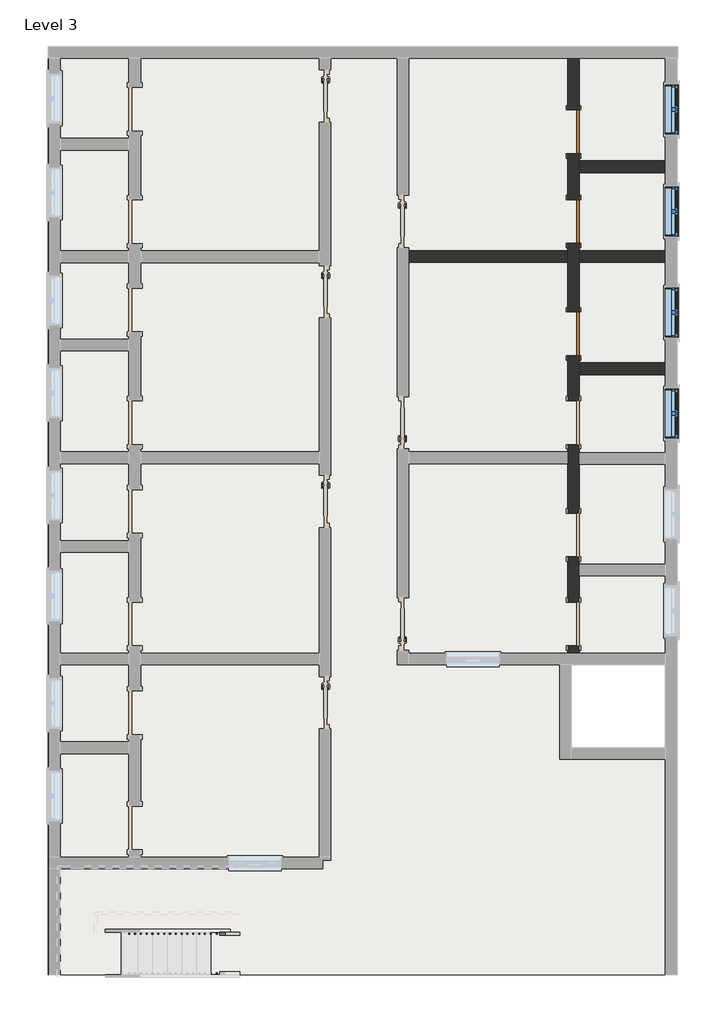
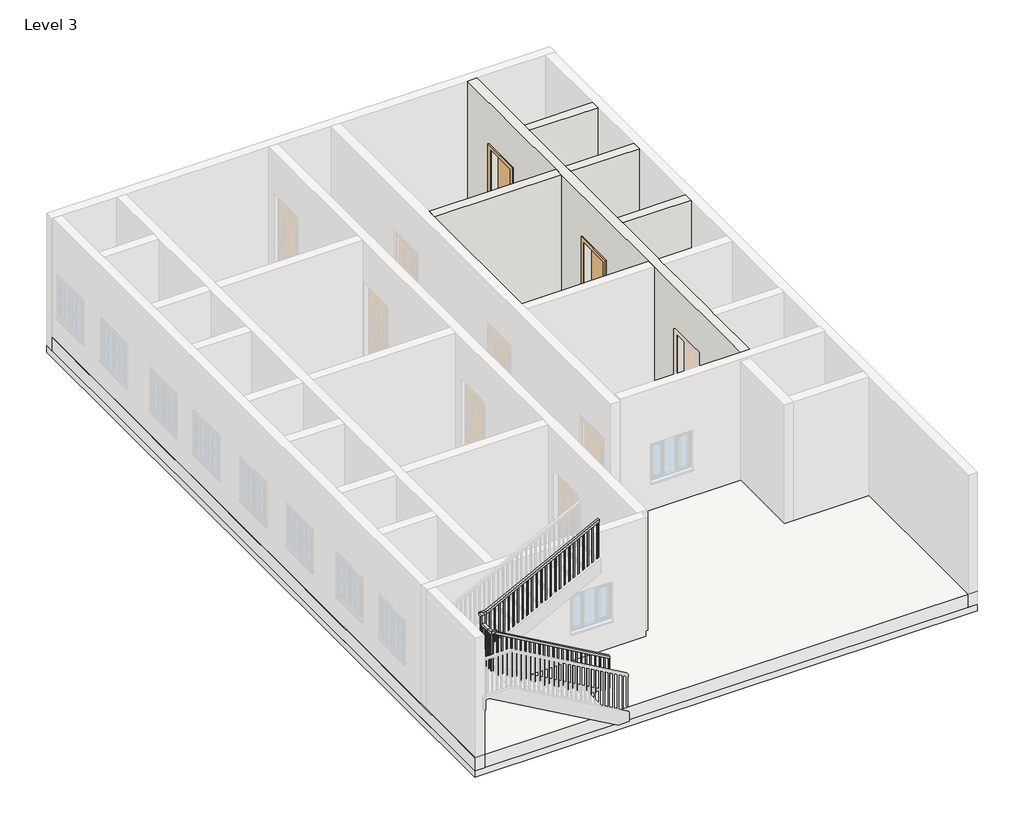
# One storey, part 2 of 4: 5 walls, 4 windows, 3 doors, 1 railing, 1 roof, 1 slab.
"""IFC4 building model written with IfcOpenShell, lengths in millimetres."""

from ifc_helpers import new_model, si_unit, frame, origin, place, context, project, spatial, polyline, outline, extrude, faceted_brep, transform, mapped, element, save
from components import door_53b1b562, window_c29befe5

model = new_model("IFC4")

# Units and contexts
model_context = context("Model", 3, world=origin())
ifc_project = project(units=[si_unit("LENGTHUNIT", "METRE", prefix="MILLI")], contexts=[model_context])

# Site, building, storey
site = spatial("IfcSite", under=ifc_project)
building = spatial("IfcBuilding", under=site)
storey = spatial("IfcBuildingStorey", under=building, Name="Level 3", Elevation=6096.0)

# Doors
placement = place(None, origin())
door_shape = door_53b1b562(model_context)
element("IfcDoor", 1, ObjectType="Single-Flush : 30\" x 80\"", at=placement, inside=storey, context=model_context, shape_type="MappedRepresentation", body=[
    mapped(door_shape, transform((2695.5891134, 6512.9399728, 6096.0), x_axis=(0.0, 1.0, 0.0), y_axis=(-1.0, 0.0, 0.0), z_axis=(0.0, 0.0, 1.0))),
])
element("IfcDoor", 2, ObjectType="Single-Flush : 30\" x 80\"", at=placement, inside=storey, context=model_context, shape_type="MappedRepresentation", body=[
    mapped(door_shape, transform((2695.5891134, 4950.8399728, 6096.0), x_axis=(0.0, 1.0, 0.0), y_axis=(-1.0, 0.0, 0.0), z_axis=(0.0, 0.0, 1.0))),
])
element("IfcDoor", 3, ObjectType="Single-Flush : 30\" x 80\"", at=placement, inside=storey, context=model_context, shape_type="MappedRepresentation", body=[
    mapped(door_shape, transform((2695.5891134, 2995.0399728, 6096.0), x_axis=(0.0, 1.0, 0.0), y_axis=(-1.0, 0.0, 0.0), z_axis=(0.0, 0.0, 1.0))),
])

# Railing
element("IfcRailing", 4, ObjectType="Handrail - Rectangular", at=placement, inside=storey, context=model_context, shape_type="SolidModel", body=[
    faceted_brep([(-3117.2664982, -7482.4600272, 7155.5428571), (-3117.2664982, -7482.4600272, 7097.0339009), (-3117.2664982, -7431.6600272, 7097.0339009), (-3117.2664982, -7431.6600272, 7155.5428571), (-5581.0664982, -7482.4600272, 8563.4285714), (-5631.8664982, -7482.4600272, 8533.9481866), (-5631.8664982, -7431.6600272, 8533.9481866), (-5581.0664982, -7431.6600272, 8563.4285714), (-5581.0664982, -7482.4600272, 8606.9714286), (-5631.8664982, -7482.4600272, 8556.1714286), (-5631.8664982, -7431.6600272, 8556.1714286), (-5581.0664982, -7431.6600272, 8606.9714286), (-5708.0664982, -7482.4600272, 8606.9714286), (-5708.0664982, -7482.4600272, 8556.1714286), (-5657.2664982, -7431.6600272, 8556.1714286), (-5657.2664982, -7431.6600272, 8606.9714286), (-5708.0664982, -7355.4600272, 8606.9714286), (-5708.0664982, -7355.4600272, 8556.1714286), (-5657.2664982, -7355.4600272, 8556.1714286), (-5657.2664982, -7355.4600272, 8606.9714286), (-5708.0664982, -7152.2600272, 8606.9714286), (-5708.0664982, -7101.4600272, 8556.1714286), (-5657.2664982, -7101.4600272, 8556.1714286), (-5657.2664982, -7152.2600272, 8606.9714286), (-5708.0664982, -7152.2600272, 8791.3028571), (-5708.0664982, -7101.4600272, 8740.5028571), (-5657.2664982, -7101.4600272, 8740.5028571), (-5657.2664982, -7152.2600272, 8791.3028571), (-5708.0664982, -7025.2600272, 8791.3028571), (-5708.0664982, -7025.2600272, 8740.5028571), (-5657.2664982, -7076.0600272, 8740.5028571), (-5657.2664982, -7076.0600272, 8791.3028571), (-5581.0664982, -7025.2600272, 8791.3028571), (-5568.769124, -7025.2600272, 8740.5028571), (-5568.769124, -7076.0600272, 8740.5028571), (-5581.0664982, -7076.0600272, 8791.3028571), (-3117.2664982, -7025.2600272, 10058.4), (-3117.2664982, -7076.0600272, 10058.4), (-3117.2664982, -7076.0600272, 10001.2756361), (-3117.2664982, -7025.2600272, 10001.2756361)], [[[0, 1, 2, 3]], [[1, 0, 4, 5]], [[2, 1, 5, 6]], [[3, 2, 6, 7]], [[0, 3, 7, 4]], [[5, 4, 8, 9]], [[6, 5, 9, 10]], [[7, 6, 10, 11]], [[4, 7, 11, 8]], [[9, 8, 12, 13]], [[10, 9, 13, 14]], [[11, 10, 14, 15]], [[8, 11, 15, 12]], [[13, 12, 16, 17]], [[14, 13, 17, 18]], [[15, 14, 18, 19]], [[12, 15, 19, 16]], [[17, 16, 20, 21]], [[18, 17, 21, 22]], [[19, 18, 22, 23]], [[16, 19, 23, 20]], [[21, 20, 24, 25]], [[22, 21, 25, 26]], [[23, 22, 26, 27]], [[20, 23, 27, 24]], [[25, 24, 28, 29]], [[26, 25, 29, 30]], [[27, 26, 30, 31]], [[24, 27, 31, 28]], [[29, 28, 32, 33]], [[30, 29, 33, 34]], [[31, 30, 34, 35]], [[28, 31, 35, 32]], [[36, 37, 38, 39]], [[33, 32, 36, 39]], [[34, 33, 39, 38]], [[35, 34, 38, 37]], [[32, 35, 37, 36]]]),
    extrude(outline(polyline([(9993.1113504, -3133.1414982), (9983.3142076, -3152.1914982), (8998.8571429, -3152.1914982), (8998.8571429, -3133.1414982), (9993.1113504, -3133.1414982)])), frame((0.0, -7060.1850272, 0.0), z_axis=(0.0, 1.0, 0.0), x_axis=(0.0, 0.0, 1.0)), (0.0, 0.0, 1.0), 19.05),
    extrude(outline(polyline([(9940.8599218, -3234.7414982), (9931.062779, -3253.7914982), (8998.8571429, -3253.7914982), (8998.8571429, -3234.7414982), (9940.8599218, -3234.7414982)])), frame((0.0, -7060.1850272, 0.0), z_axis=(0.0, 1.0, 0.0), x_axis=(0.0, 0.0, 1.0)), (0.0, 0.0, 1.0), 19.05),
    extrude(outline(polyline([(9888.6084933, -3336.3414982), (9878.8113504, -3355.3914982), (8998.8571429, -3355.3914982), (8998.8571429, -3336.3414982), (9888.6084933, -3336.3414982)])), frame((0.0, -7060.1850272, 0.0), z_axis=(0.0, 1.0, 0.0), x_axis=(0.0, 0.0, 1.0)), (0.0, 0.0, 1.0), 19.05),
    extrude(outline(polyline([(9836.3570647, -3437.9414982), (9826.5599218, -3456.9914982), (8853.7142857, -3456.9914982), (8853.7142857, -3437.9414982), (9836.3570647, -3437.9414982)])), frame((0.0, -7060.1850272, 0.0), z_axis=(0.0, 1.0, 0.0), x_axis=(0.0, 0.0, 1.0)), (0.0, 0.0, 1.0), 19.05),
    extrude(outline(polyline([(9784.1056361, -3539.5414982), (9774.3084933, -3558.5914982), (8853.7142857, -3558.5914982), (8853.7142857, -3539.5414982), (9784.1056361, -3539.5414982)])), frame((0.0, -7060.1850272, 0.0), z_axis=(0.0, 1.0, 0.0), x_axis=(0.0, 0.0, 1.0)), (0.0, 0.0, 1.0), 19.05),
    extrude(outline(polyline([(9731.8542076, -3641.1414982), (9722.0570647, -3660.1914982), (8708.5714286, -3660.1914982), (8708.5714286, -3641.1414982), (9731.8542076, -3641.1414982)])), frame((0.0, -7060.1850272, 0.0), z_axis=(0.0, 1.0, 0.0), x_axis=(0.0, 0.0, 1.0)), (0.0, 0.0, 1.0), 19.05),
    extrude(outline(polyline([(9679.602779, -3742.7414982), (9669.8056361, -3761.7914982), (8708.5714286, -3761.7914982), (8708.5714286, -3742.7414982), (9679.602779, -3742.7414982)])), frame((0.0, -7060.1850272, 0.0), z_axis=(0.0, 1.0, 0.0), x_axis=(0.0, 0.0, 1.0)), (0.0, 0.0, 1.0), 19.05),
    extrude(outline(polyline([(9627.3513504, -3844.3414982), (9617.5542076, -3863.3914982), (8708.5714286, -3863.3914982), (8708.5714286, -3844.3414982), (9627.3513504, -3844.3414982)])), frame((0.0, -7060.1850272, 0.0), z_axis=(0.0, 1.0, 0.0), x_axis=(0.0, 0.0, 1.0)), (0.0, 0.0, 1.0), 19.05),
    extrude(outline(polyline([(9575.0999218, -3945.9414982), (9565.302779, -3964.9914982), (8708.5714286, -3964.9914982), (8708.5714286, -3945.9414982), (9575.0999218, -3945.9414982)])), frame((0.0, -7060.1850272, 0.0), z_axis=(0.0, 1.0, 0.0), x_axis=(0.0, 0.0, 1.0)), (0.0, 0.0, 1.0), 19.05),
    extrude(outline(polyline([(9522.8484933, -4047.5414982), (9513.0513504, -4066.5914982), (8708.5714286, -4066.5914982), (8708.5714286, -4047.5414982), (9522.8484933, -4047.5414982)])), frame((0.0, -7060.1850272, 0.0), z_axis=(0.0, 1.0, 0.0), x_axis=(0.0, 0.0, 1.0)), (0.0, 0.0, 1.0), 19.05),
    extrude(outline(polyline([(9470.5970647, -4149.1414982), (9460.7999218, -4168.1914982), (8563.4285714, -4168.1914982), (8563.4285714, -4149.1414982), (9470.5970647, -4149.1414982)])), frame((0.0, -7060.1850272, 0.0), z_axis=(0.0, 1.0, 0.0), x_axis=(0.0, 0.0, 1.0)), (0.0, 0.0, 1.0), 19.05),
    extrude(outline(polyline([(9418.3456361, -4250.7414982), (9408.5484933, -4269.7914982), (8563.4285714, -4269.7914982), (8563.4285714, -4250.7414982), (9418.3456361, -4250.7414982)])), frame((0.0, -7060.1850272, 0.0), z_axis=(0.0, 1.0, 0.0), x_axis=(0.0, 0.0, 1.0)), (0.0, 0.0, 1.0), 19.05),
    extrude(outline(polyline([(9366.0942076, -4352.3414982), (9356.2970647, -4371.3914982), (8563.4285714, -4371.3914982), (8563.4285714, -4352.3414982), (9366.0942076, -4352.3414982)])), frame((0.0, -7060.1850272, 0.0), z_axis=(0.0, 1.0, 0.0), x_axis=(0.0, 0.0, 1.0)), (0.0, 0.0, 1.0), 19.05),
    extrude(outline(polyline([(9313.842779, -4453.9414982), (9304.0456361, -4472.9914982), (8418.2857143, -4472.9914982), (8418.2857143, -4453.9414982), (9313.842779, -4453.9414982)])), frame((0.0, -7060.1850272, 0.0), z_axis=(0.0, 1.0, 0.0), x_axis=(0.0, 0.0, 1.0)), (0.0, 0.0, 1.0), 19.05),
    extrude(outline(polyline([(9261.5913504, -4555.5414982), (9251.7942076, -4574.5914982), (8418.2857143, -4574.5914982), (8418.2857143, -4555.5414982), (9261.5913504, -4555.5414982)])), frame((0.0, -7060.1850272, 0.0), z_axis=(0.0, 1.0, 0.0), x_axis=(0.0, 0.0, 1.0)), (0.0, 0.0, 1.0), 19.05),
    extrude(outline(polyline([(9209.3399218, -4657.1414982), (9199.542779, -4676.1914982), (8273.1428571, -4676.1914982), (8273.1428571, -4657.1414982), (9209.3399218, -4657.1414982)])), frame((0.0, -7060.1850272, 0.0), z_axis=(0.0, 1.0, 0.0), x_axis=(0.0, 0.0, 1.0)), (0.0, 0.0, 1.0), 19.05),
    extrude(outline(polyline([(9157.0884933, -4758.7414982), (9147.2913504, -4777.7914982), (8273.1428571, -4777.7914982), (8273.1428571, -4758.7414982), (9157.0884933, -4758.7414982)])), frame((0.0, -7060.1850272, 0.0), z_axis=(0.0, 1.0, 0.0), x_axis=(0.0, 0.0, 1.0)), (0.0, 0.0, 1.0), 19.05),
    extrude(outline(polyline([(9104.8370647, -4860.3414982), (9095.0399218, -4879.3914982), (8273.1428571, -4879.3914982), (8273.1428571, -4860.3414982), (9104.8370647, -4860.3414982)])), frame((0.0, -7060.1850272, 0.0), z_axis=(0.0, 1.0, 0.0), x_axis=(0.0, 0.0, 1.0)), (0.0, 0.0, 1.0), 19.05),
    extrude(outline(polyline([(9052.5856361, -4961.9414982), (9042.7884933, -4980.9914982), (8128.0, -4980.9914982), (8128.0, -4961.9414982), (9052.5856361, -4961.9414982)])), frame((0.0, -7060.1850272, 0.0), z_axis=(0.0, 1.0, 0.0), x_axis=(0.0, 0.0, 1.0)), (0.0, 0.0, 1.0), 19.05),
    extrude(outline(polyline([(9000.3342076, -5063.5414982), (8990.5370647, -5082.5914982), (8128.0, -5082.5914982), (8128.0, -5063.5414982), (9000.3342076, -5063.5414982)])), frame((0.0, -7060.1850272, 0.0), z_axis=(0.0, 1.0, 0.0), x_axis=(0.0, 0.0, 1.0)), (0.0, 0.0, 1.0), 19.05),
    extrude(outline(polyline([(8948.082779, -5165.1414982), (8938.2856361, -5184.1914982), (7982.8571429, -5184.1914982), (7982.8571429, -5165.1414982), (8948.082779, -5165.1414982)])), frame((0.0, -7060.1850272, 0.0), z_axis=(0.0, 1.0, 0.0), x_axis=(0.0, 0.0, 1.0)), (0.0, 0.0, 1.0), 19.05),
    extrude(outline(polyline([(8895.8313504, -5266.7414982), (8886.0342076, -5285.7914982), (7982.8571429, -5285.7914982), (7982.8571429, -5266.7414982), (8895.8313504, -5266.7414982)])), frame((0.0, -7060.1850272, 0.0), z_axis=(0.0, 1.0, 0.0), x_axis=(0.0, 0.0, 1.0)), (0.0, 0.0, 1.0), 19.05),
    extrude(outline(polyline([(8843.5799218, -5368.3414982), (8833.782779, -5387.3914982), (7982.8571429, -5387.3914982), (7982.8571429, -5368.3414982), (8843.5799218, -5368.3414982)])), frame((0.0, -7060.1850272, 0.0), z_axis=(0.0, 1.0, 0.0), x_axis=(0.0, 0.0, 1.0)), (0.0, 0.0, 1.0), 19.05),
    extrude(outline(polyline([(8791.3284933, -5469.9414982), (8781.5313504, -5488.9914982), (7837.7142857, -5488.9914982), (7837.7142857, -5469.9414982), (8791.3284933, -5469.9414982)])), frame((0.0, -7060.1850272, 0.0), z_axis=(0.0, 1.0, 0.0), x_axis=(0.0, 0.0, 1.0)), (0.0, 0.0, 1.0), 19.05),
    extrude(outline(polyline([(8739.0770647, -5571.5414982), (8729.2799218, -5590.5914982), (7837.7142857, -5590.5914982), (7837.7142857, -5571.5414982), (8739.0770647, -5571.5414982)])), frame((0.0, -7060.1850272, 0.0), z_axis=(0.0, 1.0, 0.0), x_axis=(0.0, 0.0, 1.0)), (0.0, 0.0, 1.0), 19.05),
    extrude(outline(polyline([(-5673.1414982, -7161.7850272), (-5692.1914982, -7161.7850272), (-5692.1914982, -7142.7350272), (-5673.1414982, -7142.7350272), (-5673.1414982, -7161.7850272)])), frame((0.0, 0.0, 7692.5714286), z_axis=(0.0, 0.0, 1.0), x_axis=(1.0, 0.0, 0.0)), (0.0, 0.0, 1.0), 863.6),
    extrude(outline(polyline([(-5673.1414982, -7263.3850272), (-5692.1914982, -7263.3850272), (-5692.1914982, -7244.3350272), (-5673.1414982, -7244.3350272), (-5673.1414982, -7263.3850272)])), frame((0.0, 0.0, 7692.5714286), z_axis=(0.0, 0.0, 1.0), x_axis=(1.0, 0.0, 0.0)), (0.0, 0.0, 1.0), 863.6),
    extrude(outline(polyline([(-5673.1414982, -7364.9850272), (-5692.1914982, -7364.9850272), (-5692.1914982, -7345.9350272), (-5673.1414982, -7345.9350272), (-5673.1414982, -7364.9850272)])), frame((0.0, 0.0, 7692.5714286), z_axis=(0.0, 0.0, 1.0), x_axis=(1.0, 0.0, 0.0)), (0.0, 0.0, 1.0), 863.6),
    extrude(outline(polyline([(-5647.7414982, -7447.5350272), (-5647.7414982, -7466.5850272), (-5666.7914982, -7466.5850272), (-5666.7914982, -7447.5350272), (-5647.7414982, -7447.5350272)])), frame((0.0, 0.0, 7692.5714286), z_axis=(0.0, 0.0, 1.0), x_axis=(1.0, 0.0, 0.0)), (0.0, 0.0, 1.0), 863.6),
    extrude(outline(polyline([(8484.9624723, -5546.1414982), (8495.8481866, -5565.1914982), (7547.4285714, -5565.1914982), (7547.4285714, -5546.1414982), (8484.9624723, -5546.1414982)])), frame((0.0, -7466.5850272, 0.0), z_axis=(0.0, 1.0, 0.0), x_axis=(0.0, 0.0, 1.0)), (0.0, 0.0, 1.0), 19.05),
    extrude(outline(polyline([(8426.9053295, -5444.5414982), (8437.7910438, -5463.5914982), (7547.4285714, -5463.5914982), (7547.4285714, -5444.5414982), (8426.9053295, -5444.5414982)])), frame((0.0, -7466.5850272, 0.0), z_axis=(0.0, 1.0, 0.0), x_axis=(0.0, 0.0, 1.0)), (0.0, 0.0, 1.0), 19.05),
    extrude(outline(polyline([(8368.8481866, -5342.9414982), (8379.7339009, -5361.9914982), (7402.2857143, -5361.9914982), (7402.2857143, -5342.9414982), (8368.8481866, -5342.9414982)])), frame((0.0, -7466.5850272, 0.0), z_axis=(0.0, 1.0, 0.0), x_axis=(0.0, 0.0, 1.0)), (0.0, 0.0, 1.0), 19.05),
    extrude(outline(polyline([(8310.7910438, -5241.3414982), (8321.6767581, -5260.3914982), (7402.2857143, -5260.3914982), (7402.2857143, -5241.3414982), (8310.7910438, -5241.3414982)])), frame((0.0, -7466.5850272, 0.0), z_axis=(0.0, 1.0, 0.0), x_axis=(0.0, 0.0, 1.0)), (0.0, 0.0, 1.0), 19.05),
    extrude(outline(polyline([(8252.7339009, -5139.7414982), (8263.6196152, -5158.7914982), (7402.2857143, -5158.7914982), (7402.2857143, -5139.7414982), (8252.7339009, -5139.7414982)])), frame((0.0, -7466.5850272, 0.0), z_axis=(0.0, 1.0, 0.0), x_axis=(0.0, 0.0, 1.0)), (0.0, 0.0, 1.0), 19.05),
    extrude(outline(polyline([(8194.6767581, -5038.1414982), (8205.5624723, -5057.1914982), (7257.1428571, -5057.1914982), (7257.1428571, -5038.1414982), (8194.6767581, -5038.1414982)])), frame((0.0, -7466.5850272, 0.0), z_axis=(0.0, 1.0, 0.0), x_axis=(0.0, 0.0, 1.0)), (0.0, 0.0, 1.0), 19.05),
    extrude(outline(polyline([(8136.6196152, -4936.5414982), (8147.5053295, -4955.5914982), (7257.1428571, -4955.5914982), (7257.1428571, -4936.5414982), (8136.6196152, -4936.5414982)])), frame((0.0, -7466.5850272, 0.0), z_axis=(0.0, 1.0, 0.0), x_axis=(0.0, 0.0, 1.0)), (0.0, 0.0, 1.0), 19.05),
    extrude(outline(polyline([(8078.5624723, -4834.9414982), (8089.4481866, -4853.9914982), (7112.0, -4853.9914982), (7112.0, -4834.9414982), (8078.5624723, -4834.9414982)])), frame((0.0, -7466.5850272, 0.0), z_axis=(0.0, 1.0, 0.0), x_axis=(0.0, 0.0, 1.0)), (0.0, 0.0, 1.0), 19.05),
    extrude(outline(polyline([(8020.5053295, -4733.3414982), (8031.3910438, -4752.3914982), (7112.0, -4752.3914982), (7112.0, -4733.3414982), (8020.5053295, -4733.3414982)])), frame((0.0, -7466.5850272, 0.0), z_axis=(0.0, 1.0, 0.0), x_axis=(0.0, 0.0, 1.0)), (0.0, 0.0, 1.0), 19.05),
    extrude(outline(polyline([(7962.4481866, -4631.7414982), (7973.3339009, -4650.7914982), (7112.0, -4650.7914982), (7112.0, -4631.7414982), (7962.4481866, -4631.7414982)])), frame((0.0, -7466.5850272, 0.0), z_axis=(0.0, 1.0, 0.0), x_axis=(0.0, 0.0, 1.0)), (0.0, 0.0, 1.0), 19.05),
    extrude(outline(polyline([(7904.3910438, -4530.1414982), (7915.2767581, -4549.1914982), (6966.8571429, -4549.1914982), (6966.8571429, -4530.1414982), (7904.3910438, -4530.1414982)])), frame((0.0, -7466.5850272, 0.0), z_axis=(0.0, 1.0, 0.0), x_axis=(0.0, 0.0, 1.0)), (0.0, 0.0, 1.0), 19.05),
    extrude(outline(polyline([(7846.3339009, -4428.5414982), (7857.2196152, -4447.5914982), (6966.8571429, -4447.5914982), (6966.8571429, -4428.5414982), (7846.3339009, -4428.5414982)])), frame((0.0, -7466.5850272, 0.0), z_axis=(0.0, 1.0, 0.0), x_axis=(0.0, 0.0, 1.0)), (0.0, 0.0, 1.0), 19.05),
    extrude(outline(polyline([(7788.2767581, -4326.9414982), (7799.1624723, -4345.9914982), (6821.7142857, -4345.9914982), (6821.7142857, -4326.9414982), (7788.2767581, -4326.9414982)])), frame((0.0, -7466.5850272, 0.0), z_axis=(0.0, 1.0, 0.0), x_axis=(0.0, 0.0, 1.0)), (0.0, 0.0, 1.0), 19.05),
    extrude(outline(polyline([(7730.2196152, -4225.3414982), (7741.1053295, -4244.3914982), (6821.7142857, -4244.3914982), (6821.7142857, -4225.3414982), (7730.2196152, -4225.3414982)])), frame((0.0, -7466.5850272, 0.0), z_axis=(0.0, 1.0, 0.0), x_axis=(0.0, 0.0, 1.0)), (0.0, 0.0, 1.0), 19.05),
    extrude(outline(polyline([(7672.1624723, -4123.7414982), (7683.0481866, -4142.7914982), (6821.7142857, -4142.7914982), (6821.7142857, -4123.7414982), (7672.1624723, -4123.7414982)])), frame((0.0, -7466.5850272, 0.0), z_axis=(0.0, 1.0, 0.0), x_axis=(0.0, 0.0, 1.0)), (0.0, 0.0, 1.0), 19.05),
    extrude(outline(polyline([(7614.1053295, -4022.1414982), (7624.9910438, -4041.1914982), (6676.5714286, -4041.1914982), (6676.5714286, -4022.1414982), (7614.1053295, -4022.1414982)])), frame((0.0, -7466.5850272, 0.0), z_axis=(0.0, 1.0, 0.0), x_axis=(0.0, 0.0, 1.0)), (0.0, 0.0, 1.0), 19.05),
    extrude(outline(polyline([(7556.0481866, -3920.5414982), (7566.9339009, -3939.5914982), (6676.5714286, -3939.5914982), (6676.5714286, -3920.5414982), (7556.0481866, -3920.5414982)])), frame((0.0, -7466.5850272, 0.0), z_axis=(0.0, 1.0, 0.0), x_axis=(0.0, 0.0, 1.0)), (0.0, 0.0, 1.0), 19.05),
    extrude(outline(polyline([(7497.9910438, -3818.9414982), (7508.8767581, -3837.9914982), (6531.4285714, -3837.9914982), (6531.4285714, -3818.9414982), (7497.9910438, -3818.9414982)])), frame((0.0, -7466.5850272, 0.0), z_axis=(0.0, 1.0, 0.0), x_axis=(0.0, 0.0, 1.0)), (0.0, 0.0, 1.0), 19.05),
    extrude(outline(polyline([(7439.9339009, -3717.3414982), (7450.8196152, -3736.3914982), (6531.4285714, -3736.3914982), (6531.4285714, -3717.3414982), (7439.9339009, -3717.3414982)])), frame((0.0, -7466.5850272, 0.0), z_axis=(0.0, 1.0, 0.0), x_axis=(0.0, 0.0, 1.0)), (0.0, 0.0, 1.0), 19.05),
    extrude(outline(polyline([(7381.8767581, -3615.7414982), (7392.7624723, -3634.7914982), (6531.4285714, -3634.7914982), (6531.4285714, -3615.7414982), (7381.8767581, -3615.7414982)])), frame((0.0, -7466.5850272, 0.0), z_axis=(0.0, 1.0, 0.0), x_axis=(0.0, 0.0, 1.0)), (0.0, 0.0, 1.0), 19.05),
    extrude(outline(polyline([(7323.8196152, -3514.1414982), (7334.7053295, -3533.1914982), (6386.2857143, -3533.1914982), (6386.2857143, -3514.1414982), (7323.8196152, -3514.1414982)])), frame((0.0, -7466.5850272, 0.0), z_axis=(0.0, 1.0, 0.0), x_axis=(0.0, 0.0, 1.0)), (0.0, 0.0, 1.0), 19.05),
    extrude(outline(polyline([(7265.7624723, -3412.5414982), (7276.6481866, -3431.5914982), (6386.2857143, -3431.5914982), (6386.2857143, -3412.5414982), (7265.7624723, -3412.5414982)])), frame((0.0, -7466.5850272, 0.0), z_axis=(0.0, 1.0, 0.0), x_axis=(0.0, 0.0, 1.0)), (0.0, 0.0, 1.0), 19.05),
    extrude(outline(polyline([(7207.7053295, -3310.9414982), (7218.5910438, -3329.9914982), (6241.1428571, -3329.9914982), (6241.1428571, -3310.9414982), (7207.7053295, -3310.9414982)])), frame((0.0, -7466.5850272, 0.0), z_axis=(0.0, 1.0, 0.0), x_axis=(0.0, 0.0, 1.0)), (0.0, 0.0, 1.0), 19.05),
    extrude(outline(polyline([(7149.6481866, -3209.3414982), (7160.5339009, -3228.3914982), (6241.1428571, -3228.3914982), (6241.1428571, -3209.3414982), (7149.6481866, -3209.3414982)])), frame((0.0, -7466.5850272, 0.0), z_axis=(0.0, 1.0, 0.0), x_axis=(0.0, 0.0, 1.0)), (0.0, 0.0, 1.0), 19.05),
    extrude(outline(polyline([(-5673.1414982, -7060.1850272), (-5692.1914982, -7060.1850272), (-5692.1914982, -7041.1350272), (-5673.1414982, -7041.1350272), (-5673.1414982, -7060.1850272)])), frame((0.0, 0.0, 7692.5714286), z_axis=(0.0, 0.0, 1.0), x_axis=(1.0, 0.0, 0.0)), (0.0, 0.0, 1.0), 1047.9314286),
    extrude(outline(polyline([(-5673.1414982, -7447.5350272), (-5673.1414982, -7466.5850272), (-5692.1914982, -7466.5850272), (-5692.1914982, -7447.5350272), (-5673.1414982, -7447.5350272)])), frame((0.0, 0.0, 7692.5714286), z_axis=(0.0, 0.0, 1.0), x_axis=(1.0, 0.0, 0.0)), (0.0, 0.0, 1.0), 863.6),
    extrude(outline(polyline([(10001.2756361, -3117.2664982), (9991.4784933, -3136.3164982), (8998.8571429, -3136.3164982), (8998.8571429, -3117.2664982), (10001.2756361, -3117.2664982)])), frame((0.0, -7060.1850272, 0.0), z_axis=(0.0, 1.0, 0.0), x_axis=(0.0, 0.0, 1.0)), (0.0, 0.0, 1.0), 19.05),
    extrude(outline(polyline([(7097.0339009, -3117.2664982), (7107.9196152, -3136.3164982), (6241.1428571, -3136.3164982), (6241.1428571, -3117.2664982), (7097.0339009, -3117.2664982)])), frame((0.0, -7466.5850272, 0.0), z_axis=(0.0, 1.0, 0.0), x_axis=(0.0, 0.0, 1.0)), (0.0, 0.0, 1.0), 19.05),
])

# Roof
element("IfcRoof", 5, ObjectType="Generic - 12\"", at=placement, inside=storey, context=model_context, shape_type="SweptSolid", body=[
    extrude(outline(polyline([(-6461.1108866, -8168.2600272), (-6461.1108866, 7998.8399728), (4498.9891134, 7998.8399728), (4498.9891134, -8168.2600272), (-6461.1108866, -8168.2600272)]), holes=[polyline([(4295.7891134, -2770.7600272), (2657.4891134, -2770.7600272), (2657.4891134, -4218.5600272), (4295.7891134, -4218.5600272), (4295.7891134, -2770.7600272)])]), frame((0.0, 0.0, 6096.0), z_axis=(0.0, 0.0, 1.0), x_axis=(1.0, 0.0, 0.0)), (0.0, 0.0, 1.0), 304.8),
])

# Slab
element("IfcSlab", 6, ObjectType="Generic - 12\"", at=placement, inside=storey, context=model_context, shape_type="SweptSolid", body=[
    extrude(outline(polyline([(4498.9891134, 7998.8399728), (4498.9891134, -8168.2600272), (-6461.1108866, -8168.2600272), (-6461.1108866, 7998.8399728), (4498.9891134, 7998.8399728)]), holes=[polyline([(4295.7891134, -2770.7600272), (2657.4891134, -2770.7600272), (2657.4891134, -4218.5600272), (4295.7891134, -4218.5600272), (4295.7891134, -2770.7600272)])]), frame((0.0, 0.0, 5943.6), z_axis=(0.0, 0.0, 1.0), x_axis=(1.0, 0.0, 0.0)), (0.0, 0.0, 1.0), 152.4),
])

# Walls
element("IfcWall", 7, ObjectType="4.5\" p", at=placement, inside=storey, context=model_context, shape_type="Brep", body=[
    faceted_brep([(2593.9891134, -2440.5600272, 8128.0), (2593.9891134, -2440.5600272, 6096.0), (2593.9891134, -2567.5600272, 6096.0), (2593.9891134, -2567.5600272, 9144.0), (2593.9891134, 734.4399728, 9144.0), (2593.9891134, 937.6399728, 9144.0), (2593.9891134, 4239.6399728, 9144.0), (2593.9891134, 4442.8399728, 9144.0), (2593.9891134, 7795.6399728, 9144.0), (2593.9891134, 7795.6399728, 6096.0), (2593.9891134, 6893.9399728, 6096.0), (2593.9891134, 6893.9399728, 8128.0), (2593.9891134, 6131.9399728, 8128.0), (2593.9891134, 6131.9399728, 6096.0), (2593.9891134, 5331.8399728, 6096.0), (2593.9891134, 5331.8399728, 8128.0), (2593.9891134, 4569.8399728, 8128.0), (2593.9891134, 4569.8399728, 6096.0), (2593.9891134, 4442.8399728, 6096.0), (2593.9891134, 4239.6399728, 6096.0), (2593.9891134, 3376.0399728, 6096.0), (2593.9891134, 3376.0399728, 8128.0), (2593.9891134, 2614.0399728, 8128.0), (2593.9891134, 2614.0399728, 6096.0), (2593.9891134, 1826.6399728, 6096.0), (2593.9891134, 1826.6399728, 8128.0), (2593.9891134, 1064.6399728, 8128.0), (2593.9891134, 1064.6399728, 6096.0), (2593.9891134, 937.6399728, 6096.0), (2593.9891134, 734.4399728, 6096.0), (2593.9891134, -129.1600272, 6096.0), (2593.9891134, -129.1600272, 8128.0), (2593.9891134, -891.1600272, 8128.0), (2593.9891134, -891.1600272, 6096.0), (2593.9891134, -1678.5600272, 6096.0), (2593.9891134, -1678.5600272, 8128.0), (2797.1891134, -2567.5600272, 6096.0), (2797.1891134, -2440.5600272, 6096.0), (2797.1891134, -2440.5600272, 8128.0), (2797.1891134, -1678.5600272, 8128.0), (2797.1891134, -1678.5600272, 6096.0), (2797.1891134, -1221.3600272, 6096.0), (2797.1891134, -1018.1600272, 6096.0), (2797.1891134, -891.1600272, 6096.0), (2797.1891134, -891.1600272, 8128.0), (2797.1891134, -129.1600272, 8128.0), (2797.1891134, -129.1600272, 6096.0), (2797.1891134, 721.7399728, 6096.0), (2797.1891134, 924.9399728, 6096.0), (2797.1891134, 1064.6399728, 6096.0), (2797.1891134, 1064.6399728, 8128.0), (2797.1891134, 1826.6399728, 8128.0), (2797.1891134, 1826.6399728, 6096.0), (2797.1891134, 2283.8399728, 6096.0), (2797.1891134, 2487.0399728, 6096.0), (2797.1891134, 2614.0399728, 6096.0), (2797.1891134, 2614.0399728, 8128.0), (2797.1891134, 3376.0399728, 8128.0), (2797.1891134, 3376.0399728, 6096.0), (2797.1891134, 4239.6399728, 6096.0), (2797.1891134, 4442.8399728, 6096.0), (2797.1891134, 4569.8399728, 6096.0), (2797.1891134, 4569.8399728, 8128.0), (2797.1891134, 5331.8399728, 8128.0), (2797.1891134, 5331.8399728, 6096.0), (2797.1891134, 5801.7399728, 6096.0), (2797.1891134, 6004.9399728, 6096.0), (2797.1891134, 6131.9399728, 6096.0), (2797.1891134, 6131.9399728, 8128.0), (2797.1891134, 6893.9399728, 8128.0), (2797.1891134, 6893.9399728, 6096.0), (2797.1891134, 7795.6399728, 6096.0), (2797.1891134, 7795.6399728, 9144.0), (2797.1891134, 6004.9399728, 9144.0), (2797.1891134, 5801.7399728, 9144.0), (2797.1891134, 4442.8399728, 9144.0), (2797.1891134, 4239.6399728, 9144.0), (2797.1891134, 2487.0399728, 9144.0), (2797.1891134, 2283.8399728, 9144.0), (2797.1891134, 924.9399728, 9144.0), (2797.1891134, 721.7399728, 9144.0), (2797.1891134, -1018.1600272, 9144.0), (2797.1891134, -1221.3600272, 9144.0), (2797.1891134, -2567.5600272, 9144.0)], [[[0, 1, 2, 3, 4, 5, 6, 7, 8, 9, 10, 11, 12, 13, 14, 15, 16, 17, 18, 19, 20, 21, 22, 23, 24, 25, 26, 27, 28, 29, 30, 31, 32, 33, 34, 35]], [[36, 37, 38, 39, 40, 41, 42, 43, 44, 45, 46, 47, 48, 49, 50, 51, 52, 53, 54, 55, 56, 57, 58, 59, 60, 61, 62, 63, 64, 65, 66, 67, 68, 69, 70, 71, 72, 73, 74, 75, 76, 77, 78, 79, 80, 81, 82, 83]], [[71, 70, 10, 9]], [[67, 66, 65, 64, 14, 13]], [[61, 60, 59, 58, 20, 19, 18, 17]], [[55, 54, 53, 52, 24, 23]], [[30, 29, 28, 27, 49, 48, 47, 46]], [[34, 33, 43, 42, 41, 40]], [[2, 1, 37, 36]], [[8, 7, 6, 5, 4, 3, 83, 82, 81, 80, 79, 78, 77, 76, 75, 74, 73, 72]], [[9, 8, 72, 71]], [[3, 2, 36, 83]], [[11, 10, 70, 69]], [[12, 11, 69, 68]], [[13, 12, 68, 67]], [[15, 14, 64, 63]], [[16, 15, 63, 62]], [[17, 16, 62, 61]], [[21, 20, 58, 57]], [[22, 21, 57, 56]], [[23, 22, 56, 55]], [[25, 24, 52, 51]], [[26, 25, 51, 50]], [[27, 26, 50, 49]], [[44, 43, 33, 32]], [[45, 44, 32, 31]], [[46, 45, 31, 30]], [[38, 37, 1, 0]], [[39, 38, 0, 35]], [[40, 39, 35, 34]]]),
])
element("IfcWall", 8, ObjectType="4.5\" p", at=placement, inside=storey, context=model_context, shape_type="SweptSolid", body=[
    extrude(outline(polyline([(4295.7891134, 5801.7399728), (2797.1891134, 5801.7399728), (2797.1891134, 6004.9399728), (4295.7891134, 6004.9399728), (4295.7891134, 5801.7399728)])), frame((0.0, 0.0, 6096.0), z_axis=(0.0, 0.0, 1.0), x_axis=(1.0, 0.0, 0.0)), (0.0, 0.0, 1.0), 3048.0),
])
element("IfcWall", 9, ObjectType="4.5\" p", at=placement, inside=storey, context=model_context, shape_type="SweptSolid", body=[
    extrude(outline(polyline([(4295.7891134, 4239.6399728), (2797.1891134, 4239.6399728), (2797.1891134, 4442.8399728), (4295.7891134, 4442.8399728), (4295.7891134, 4239.6399728)])), frame((0.0, 0.0, 6096.0), z_axis=(0.0, 0.0, 1.0), x_axis=(1.0, 0.0, 0.0)), (0.0, 0.0, 1.0), 3048.0),
])
element("IfcWall", 10, ObjectType="4.5\" p", at=placement, inside=storey, context=model_context, shape_type="SweptSolid", body=[
    extrude(outline(polyline([(4295.7891134, 2283.8399728), (2797.1891134, 2283.8399728), (2797.1891134, 2487.0399728), (4295.7891134, 2487.0399728), (4295.7891134, 2283.8399728)])), frame((0.0, 0.0, 6096.0), z_axis=(0.0, 0.0, 1.0), x_axis=(1.0, 0.0, 0.0)), (0.0, 0.0, 1.0), 3048.0),
])
element("IfcWall", 11, ObjectType="4.5\" p", at=placement, inside=storey, context=model_context, shape_type="SweptSolid", body=[
    extrude(outline(polyline([(2593.9891134, 4239.6399728), (-174.6108866, 4239.6399728), (-174.6108866, 4442.8399728), (2593.9891134, 4442.8399728), (2593.9891134, 4239.6399728)])), frame((0.0, 0.0, 6096.0), z_axis=(0.0, 0.0, 1.0), x_axis=(1.0, 0.0, 0.0)), (0.0, 0.0, 1.0), 3048.0),
])

# Windows
window_shape = window_c29befe5(model_context)
element("IfcWindow", 12, ObjectType="Window-Casement-Double : 34\" x 36\"", at=placement, inside=storey, context=model_context, shape_type="MappedRepresentation", body=[
    mapped(window_shape, transform((4397.3891134, 1604.3899728, 6096.0), x_axis=(0.0, -1.0, 0.0), y_axis=(1.0, 0.0, 0.0), z_axis=(0.0, 0.0, 1.0))),
])
element("IfcWindow", 13, ObjectType="Window-Casement-Double : 34\" x 36\"", at=placement, inside=storey, context=model_context, shape_type="MappedRepresentation", body=[
    mapped(window_shape, transform((4397.3891134, 3363.3399728, 6096.0), x_axis=(0.0, -1.0, 0.0), y_axis=(1.0, 0.0, 0.0), z_axis=(0.0, 0.0, 1.0))),
])
element("IfcWindow", 14, ObjectType="Window-Casement-Double : 34\" x 36\"", at=placement, inside=storey, context=model_context, shape_type="MappedRepresentation", body=[
    mapped(window_shape, transform((4397.3891134, 5122.2899728, 6096.0), x_axis=(0.0, -1.0, 0.0), y_axis=(1.0, 0.0, 0.0), z_axis=(0.0, 0.0, 1.0))),
])
element("IfcWindow", 15, ObjectType="Window-Casement-Double : 34\" x 36\"", at=placement, inside=storey, context=model_context, shape_type="MappedRepresentation", body=[
    mapped(window_shape, transform((4397.3891134, 6900.2899728, 6096.0), x_axis=(0.0, -1.0, 0.0), y_axis=(1.0, 0.0, 0.0), z_axis=(0.0, 0.0, 1.0))),
])

save(model, "model.ifc")

# Revit data of these elements
# Type "Single-Flush : 30\" x 80\""
#   Type Mark = "5"
#   Construction Type Id = "MDOOR"
#   Assembly Code = "C1020"
#   Analytic Construction = "Metal"
#   Thickness = 0' - 2"
#   Heat Transfer Coefficient (U) = 0.651978 BTU/(h·ft²·°F)
#   Height = 6' - 8"
#   Trim Projection Ext = 0' - 1"
#   Trim Projection Int = 0' - 1"
#   Trim Width = 0' - 3"
#   Width = 2' - 6"
#   Define Thermal Properties by = 1
#   Define Thermal Properties by = 1
#   Door Material = Door - Panel
#   Frame Material = Door - Frame
#   Visual Light Transmittance = 0
#   Solar Heat Gain Coefficient = 0
#   Function = (empty or 0)
#   Wall Closure = (empty or 0)
# Type "Handrail - Rectangular"
#   Assembly Code = "C2010400"
#   built-in parameter 1008612 = 0.0416667 (stored number, unit not read)
#   built-in parameter 1008611 = 0.0416667 (stored number, unit not read)
#   built-in parameter 1008609 = 0.333333 (stored number, unit not read)
#   built-in parameter 1008604 = 0.166667 (stored number, unit not read)
#   built-in parameter 1008603 = 0.166667 (stored number, unit not read)
#   Railing Height = 3' - 0"
#   built-in parameter 1008630 = 2
#   built-in parameter 1008610 = 2
#   built-in parameter 1008618 = Baluster - Square : 3/4"
# Type "Generic - 12\""
#   Assembly Code = "B1020"
#   Layers, outside or top first: 1' - 0" no material (function 1)
# Type "Generic - 12\""
#   Assembly Code = "B1010"
#   Function = 0
#   Layers, outside or top first: 0' - 6" no material (function 1)
# Type "4.5\" p"
#   Assembly Code = "B2010"
#   Layers, outside or top first: 0' - 8" no material (function 1)
# Type "Window-Casement-Double : 34\" x 36\""
#   Type Mark = "14"
#   Fire Rating = "0.5h"
#   Assembly Code = "B2020100"
#   Analytic Construction = "Double glazing - domestic"
#   Frame Extension [instance default] = 0' - 0 1/4"
#   Window Inset [instance default] = 0' - 0"
#   Wall Thickness [instance default] = 0' - 6"
#   Interior Wall Closure [instance default] = 0' - 2 1/4"
#   Half Width = 1' - 5"
#   Visual Light Transmittance = 0.81
#   Thermal Resistance (R) = 1.8146 (h·ft²·°F)/BTU
#   Solar Heat Gain Coefficient = 0.76
#   Rough Width = 2' - 10 1/2"
#   Rough Height = 3' - 0 1/2"
#   Height = 3' - 0"
#   Heat Transfer Coefficient (U) = 0.5511 BTU/(h·ft²·°F)
#   Exterior Wall Closure [instance default] = 0' - 1 1/4"
#   Extension Jamb [instance default] = 0' - 2 1/4"
#   Default Sill Height = 3' - 0"
#   Width = 2' - 10"
#   Define Thermal Properties by = 0
#   Muntin Visibility = yes
#   Interior Trim Visibility [instance default] = yes
#   Exterior Trim Visibility [instance default] = yes
#   Extension Jamb Visibility [instance default] = yes
#   Interior Trim Material = Wood - Stained
#   Muntin Pattern = Muntin Pattern_2x2 : Muntin Pattern_2x2
#   Interior Trim = Trim-Window-Interior-Flat : Picture Frame
#   Interior Frame Material = Wood - Stained
#   Glass Panel Material = Glass
#   Exterior Trim Material = Clad - White
#   Exterior Trim = Trim-Window-Exterior-Flat : with Sill
#   Exterior Frame Material = Clad - White
#   Wall Closure = (empty or 0)
# Elements 1, 2, 3 (IfcDoor, "Single-Flush : 30\" x 80\"")
#   Phase Created = New Construction
#   Materials on its faces: "Door - Frame", "Door - Panel"
# Element 4 (IfcRailing, "Handrail - Rectangular")
#   Phase Created = New Construction
# Element 5 (IfcRoof, "Generic - 12\"")
#   built-in parameter 1001705 = 21 (stored number, unit not read)
#   built-in parameter 1001710 = 33615
#   Phase Created = New Construction
#   Materials on its faces: "Default Roof", "Grass", "Earth"
# Element 6 (IfcSlab, "Generic - 12\"")
#   Height Offset From Level = 0' - 0"
#   Phase Created = New Construction
#   Materials on its faces: "Default Floor", "Wood - Stained", "Earth"
# Elements 7, 8, 9, 10, 11 (IfcWall, "4.5\" p")
#   Top Offset = 0' - 0"
#   Base Offset = 0' - 0"
#   wall height = 10' - 0"
#   Phase Created = New Construction
#   Base Constraint = Level 3
#   Top Constraint = Level 4
#   Materials on its faces: "Default Wall"
# Element 12 (IfcWindow, "Window-Casement-Double : 34\" x 36\"")
#   Mark = "43"
#   Window Inset = 0' - 0"
#   Interior Wall Closure = 0' - 2 1/4"
#   Frame Extension = 0' - 0 1/4"
#   Exterior Wall Closure = 0' - 1 1/4"
#   Interior Trim Visibility = yes
#   Exterior Trim Visibility = yes
#   Phase Created = New Construction
#   Materials on its faces: "Wood - Stained", "Glass", "Clad - White"
# Element 13 (IfcWindow, "Window-Casement-Double : 34\" x 36\"")
#   Mark = "44"
#   Window Inset = 0' - 0"
#   Interior Wall Closure = 0' - 2 1/4"
#   Frame Extension = 0' - 0 1/4"
#   Exterior Wall Closure = 0' - 1 1/4"
#   Interior Trim Visibility = yes
#   Exterior Trim Visibility = yes
#   Phase Created = New Construction
#   Materials on its faces: "Wood - Stained", "Glass", "Clad - White"
# Element 14 (IfcWindow, "Window-Casement-Double : 34\" x 36\"")
#   Mark = "45"
#   Window Inset = 0' - 0"
#   Interior Wall Closure = 0' - 2 1/4"
#   Frame Extension = 0' - 0 1/4"
#   Exterior Wall Closure = 0' - 1 1/4"
#   Interior Trim Visibility = yes
#   Exterior Trim Visibility = yes
#   Phase Created = New Construction
#   Materials on its faces: "Wood - Stained", "Glass", "Clad - White"
# Element 15 (IfcWindow, "Window-Casement-Double : 34\" x 36\"")
#   Mark = "46"
#   Window Inset = 0' - 0"
#   Interior Wall Closure = 0' - 2 1/4"
#   Frame Extension = 0' - 0 1/4"
#   Exterior Wall Closure = 0' - 1 1/4"
#   Interior Trim Visibility = yes
#   Exterior Trim Visibility = yes
#   Phase Created = New Construction
#   Materials on its faces: "Wood - Stained", "Glass", "Clad - White"
# Materials
#   "Door - Panel": class "Wood", colour RGB 210 159 95, transparency 0, Cost = 0
#   "Door - Frame": colour RGB 118 70 51, transparency 0, Cost = 0
#   "Wood - Stained": class "Wood", colour RGB 224 178 126, transparency 0, Cost = 0
#   "Glass": class "Glass", colour RGB 0 128 192, transparency 0.75, Description = "Soda Lime Glass", Cost = 0
#   "Clad - White": class "Wood", colour RGB 242 242 238, transparency 0, Cost = 0
#   "Default Roof": colour RGB 88 101 114, transparency 0, Cost = 0
#   "Grass": class "Generic", colour RGB 104 137 66, transparency 0, Description = "Physical material.", Cost = 0
#   "Earth": class "Generic", colour RGB 97 75 62, transparency 0, Description = "Soil", Cost = 0
#   "Default Floor": colour RGB 128 128 128, transparency 0, Cost = 0
#   "Default Wall": colour RGB 128 128 128, transparency 0, Cost = 0
